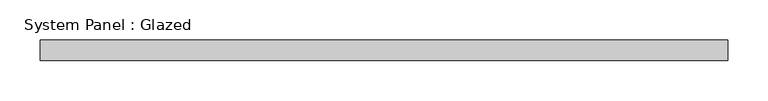
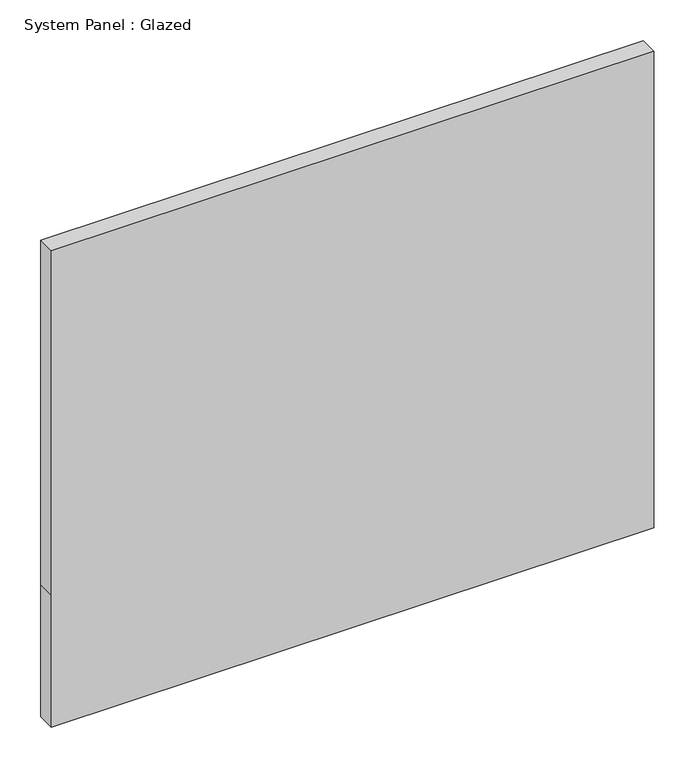
"""IFC4 building model written with IfcOpenShell, lengths in millimetres: plate geometry, System Panel : Glazed."""

from ifc_helpers import new_model, si_unit, frame, origin, place, context, project, spatial, polyline, outline, extrude, source, transform, mapped, element, save


def system_panel_glazed_ec316f56(model_context):
    return source(origin(), model_context, "Body", "SweptSolid", [
        extrude(outline(polyline([(0.0, -425.45), (0.0, 425.45), (196.85, 425.45), (711.3326807, 425.45), (711.3326807, -425.45), (196.85, -425.45), (0.0, -425.45)])), frame((0.0, 19.05, 0.0), z_axis=(0.0, 1.0, 0.0), x_axis=(0.0, 0.0, 1.0)), (0.0, 0.0, 1.0), 25.4),
    ])


if __name__ == "__main__":
    model = new_model("IFC4")
    model_context = context("Model", 3, world=origin())
    ifc_project = project(units=[si_unit("LENGTHUNIT", "METRE", prefix="MILLI")], contexts=[model_context])
    site = spatial("IfcSite", under=ifc_project)
    building = spatial("IfcBuilding", under=site)
    placement = place(None, origin())
    system_panel_glazed_shape = system_panel_glazed_ec316f56(model_context)
    element("IfcPlate", 1, ObjectType="System Panel : Glazed", at=placement, inside=building, context=model_context, shape_type="MappedRepresentation", body=[
        mapped(system_panel_glazed_shape, transform((0.0, 0.0, 0.0), x_axis=(1.0, 0.0, 0.0), y_axis=(0.0, 1.0, 0.0), z_axis=(0.0, 0.0, 1.0))),
    ])
    save(model, "model.ifc")

# Revit data of these elements
# Type "System Panel : Glazed"
#   Construction Type Id = "GSP4R"
#   Analytic Construction = "1/8 in Pilkington single glazing"
#   Visual Light Transmittance = 0.9
#   Solar Heat Gain Coefficient = 0.86
#   Heat Transfer Coefficient (U) = 1.18115 BTU/(h·ft²·°F)
#   Define Thermal Properties by = 1
# Element 1 (IfcPlate, "System Panel : Glazed")
#   Materials on its faces: "Glass"
# Materials
#   "Glass": class "Glass", colour RGB 0 128 192, transparency 0.75, Description = "Soda Lime Glass", Cost = 0
